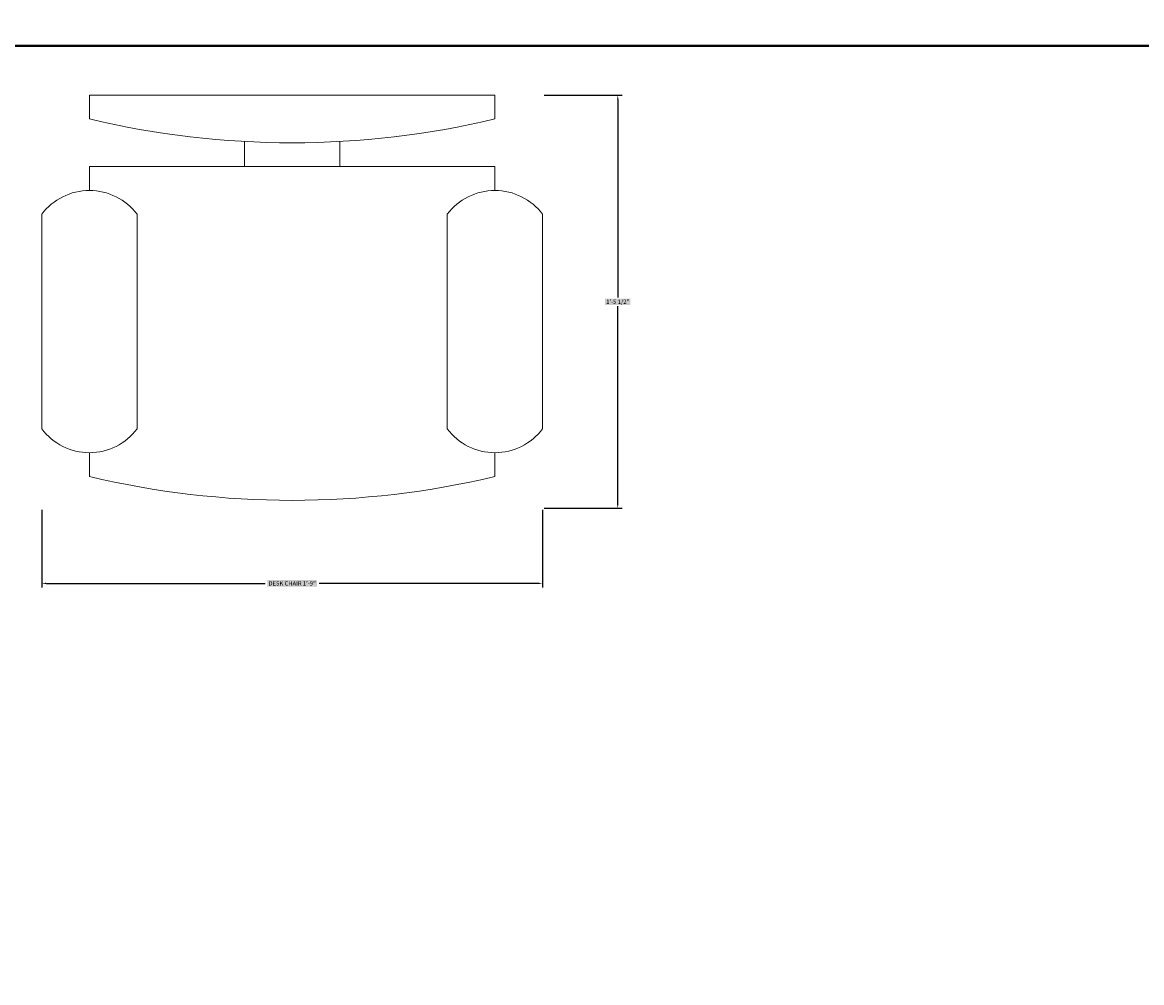
# Model space of a CAD drawing. Units: inches. Extents: x -301 to 715, y -607 to 364.
# Tile 76 of 141: x -170 to -123, y 26 to 67. Entities that reach past the tile are written whole.
import ezdxf

# ---------------------------------------------------------------- set-up
doc = ezdxf.new("R2010")
doc.units = ezdxf.units.IN
doc.header["$MEASUREMENT"] = 0
for name, color, linetype, lineweight in [('A-ANNO-DIMS', 2, 'Continuous', 18), ('A-FURN', 8, 'Continuous', 18), ('A-WALL', 3, 'Continuous', 40)]:
    doc.layers.add(name, color=color, linetype=linetype, lineweight=lineweight)
doc.styles.get("Standard").update_dxf_attribs({"font": 'arial.ttf'})
doc.dimstyles.get("Standard").update_dxf_attribs({"dimtxt": 0.18, "dimasz": 0.18, "dimexe": 0.18, "dimexo": 0.0625, "dimgap": 0.09, "dimtad": 0, "dimtih": 1, "dimtoh": 1, "dimdec": 1, "dimzin": 0, "dimdsep": 46, "dimlunit": 4, "dimtxsty": 'Standard', "dimcen": 0.09, "dimclrd": 3, "dimclre": 4, "dimclrt": 6, "dimadec": 0, "dimazin": 0, "dimtfac": 1, "dimtdec": 1, "dimtofl": 0, "dimtmove": 0, "dimatfit": 3, "dimfxl": 1, "dimtfill": 2, "dimtfillclr": 51, "dimtolj": 1, "dimtzin": 0, "dimarcsym": 0})

# ---------------------------------------------------------------- blocks, each defined once
blk = doc.blocks.new('Chair - Desk')
for p, q in [((-8.5, 0), (-8.5, -1)), ((-8.5, 0), (8.5, 0)), ((8.5, 0), (8.5, -1)), ((-2, -3), (-2, -1.9355)), ((2, -1.9576), (2, -3)), ((-8.5, -3), (-8.5, -4)), ((-8.5, -3), (8.5, -3)), ((8.5, -3), (8.5, -4)), ((-10.5, -5), (-10.5, -14)), ((-6.5, -14), (-6.5, -5)), ((6.5, -5), (6.5, -14)), ((10.5, -14), (10.5, -5)), ((-8.5, -15), (-8.5, -16)), ((8.5, -15), (8.5, -16))]:
    blk.add_line(p, q)
for centre, radius, start, end in [((0, 34.625), 36.625, 256.5803, 283.4197), ((-8.5, -6.5), 2.5, 36.8699, 143.1301), ((8.5, -6.5), 2.5, 36.8699, 143.1301), ((-8.5, -12.5), 2.5, 216.8699, 323.1301), ((8.5, -12.5), 2.5, 216.8699, 323.1301), ((0, 19.625), 36.625, 256.5803, 283.4197)]:
    blk.add_arc(centre, radius, start, end)
blk = doc.blocks.new('*D56')
at = {"layer": 'A-ANNO-DIMS', "color": 0, "lineweight": -2, "transparency": 16777216}
for p, q in [((-195.541, 65.682), (-172.295, 65.682)), ((-172.475, 60.682), (-172.475, 0.778)), ((-172.475, -62.318), (-172.475, -2.414)), ((-195.541, -67.318), (-172.295, -67.318))]:
    blk.add_line(p, q, dxfattribs=at)
at = {"layer": 'A-ANNO-DIMS', "color": 0, "transparency": 16777216}
for points in [[(-173.308, 60.682), (-171.641, 60.682), (-172.475, 65.682)], [(-173.308, -62.318), (-171.641, -62.318), (-172.475, -67.318)]]:
    blk.add_solid(points, dxfattribs=at)
at = {"layer": 'Defpoints', "color": 0, "transparency": 16777216}
for p in [(-195.603, 65.682), (-172.475, 65.682), (-195.603, -67.318)]:
    blk.add_point(p, dxfattribs=at)
at = {"layer": 'A-ANNO-DIMS', "color": 0, "transparency": 16777216, "insert": (-172.475, -0.818), "char_height": 3, "attachment_point": 5, "bg_fill": 1, "box_fill_scale": 1.25, "bg_fill_color": 51, "bg_fill_transparency": 0}
blk.add_mtext('\\A1;11\'-1"', dxfattribs=at)
blk = doc.blocks.new('*D136')
at = {"layer": 'A-ANNO-DIMS', "color": 4, "lineweight": -2, "transparency": 16777216}
for p, q in [((-169.593, 46.217), (-169.593, 42.95)), ((-148.593, 46.217), (-148.593, 42.95))]:
    blk.add_line(p, q, dxfattribs=at)
at = {"layer": 'A-ANNO-DIMS', "color": 3, "lineweight": -2, "transparency": 16777216}
for p, q in [((-169.413, 43.13), (-160.221, 43.13)), ((-148.773, 43.13), (-157.965, 43.13))]:
    blk.add_line(p, q, dxfattribs=at)
at = {"layer": 'A-ANNO-DIMS', "color": 3, "transparency": 16777216}
for points in [[(-169.413, 43.16), (-169.413, 43.1), (-169.593, 43.13)], [(-148.773, 43.16), (-148.773, 43.1), (-148.593, 43.13)]]:
    blk.add_solid(points, dxfattribs=at)
at = {"layer": 'Defpoints', "color": 0, "transparency": 16777216}
for p in [(-169.593, 46.28), (-148.593, 46.28), (-148.593, 43.13)]:
    blk.add_point(p, dxfattribs=at)
at = {"layer": 'A-ANNO-DIMS', "color": 6, "transparency": 16777216, "insert": (-159.093, 43.13), "char_height": 0.18, "attachment_point": 5, "bg_fill": 1, "box_fill_scale": 1.25, "bg_fill_color": 51, "bg_fill_transparency": 0}
blk.add_mtext('\\A1;DESK CHAIR 1\'-9"', dxfattribs=at)
blk = doc.blocks.new('*D137')
at = {"layer": 'A-ANNO-DIMS', "color": 4, "lineweight": -2, "transparency": 16777216}
for p, q in [((-148.53, 63.613), (-145.263, 63.613)), ((-148.53, 46.28), (-145.263, 46.28))]:
    blk.add_line(p, q, dxfattribs=at)
at = {"layer": 'A-ANNO-DIMS', "color": 3, "lineweight": -2, "transparency": 16777216}
for p, q in [((-145.443, 63.433), (-145.443, 55.129)), ((-145.443, 46.46), (-145.443, 54.763))]:
    blk.add_line(p, q, dxfattribs=at)
at = {"layer": 'A-ANNO-DIMS', "color": 3, "transparency": 16777216}
for points in [[(-145.473, 63.433), (-145.413, 63.433), (-145.443, 63.613)], [(-145.473, 46.46), (-145.413, 46.46), (-145.443, 46.28)]]:
    blk.add_solid(points, dxfattribs=at)
at = {"layer": 'Defpoints', "color": 0, "transparency": 16777216}
for p in [(-148.593, 63.613), (-145.443, 63.613), (-148.593, 46.28)]:
    blk.add_point(p, dxfattribs=at)
at = {"layer": 'A-ANNO-DIMS', "color": 6, "transparency": 16777216, "insert": (-145.443, 54.946), "char_height": 0.18, "attachment_point": 5, "bg_fill": 1, "box_fill_scale": 1.25, "bg_fill_color": 51, "bg_fill_transparency": 0}
blk.add_mtext('\\A1;1\'-5 1/2"', dxfattribs=at)
blk = doc.blocks.new('*D151')
at = {"layer": 'A-ANNO-DIMS', "color": 4, "lineweight": -2, "transparency": 16777216}
for p, q in [((-204.603, -223.755), (-204.603, 359.612)), ((-45.603, -214.755), (-45.603, 359.612))]:
    blk.add_line(p, q, dxfattribs=at)
at = {"layer": 'A-ANNO-DIMS', "color": 3, "lineweight": -2, "transparency": 16777216}
for p, q in [((-204.423, 359.432), (-125.494, 359.432)), ((-45.783, 359.432), (-124.713, 359.432))]:
    blk.add_line(p, q, dxfattribs=at)
at = {"layer": 'A-ANNO-DIMS', "color": 3, "transparency": 16777216}
for points in [[(-204.423, 359.462), (-204.423, 359.402), (-204.603, 359.432)], [(-45.783, 359.462), (-45.783, 359.402), (-45.603, 359.432)]]:
    blk.add_solid(points, dxfattribs=at)
at = {"layer": 'Defpoints', "color": 0, "transparency": 16777216}
for p in [(-45.603, 359.432), (-45.603, -214.818), (-204.603, -223.818)]:
    blk.add_point(p, dxfattribs=at)
at = {"layer": 'A-ANNO-DIMS', "color": 6, "transparency": 16777216, "insert": (-125.103, 359.432), "char_height": 0.18, "attachment_point": 5, "bg_fill": 1, "box_fill_scale": 1.25, "bg_fill_color": 51, "bg_fill_transparency": 0}
blk.add_mtext('\\A1;13\'-3"', dxfattribs=at)

msp = doc.modelspace()

# ---------------------------------------------------------------- linework, layer by layer
at = {"layer": 'A-WALL'}
msp.add_line((-45.603, 65.682), (-195.603, 65.682), dxfattribs=at)

# ---------------------------------------------------------------- block references
at = {"layer": 'A-FURN'}
msp.add_blockref('Chair - Desk', (-159.093, 63.613), dxfattribs=at)

# ---------------------------------------------------------------- dimensions: what is measured, and where the dimension line sits
at = {"layer": 'A-ANNO-DIMS'}
dim = msp.add_linear_dim(base=(-45.603, 359.432), p1=(-204.603, -223.818), p2=(-45.603, -214.818), dimstyle='Standard', override={"dimdec": 1, "dimlfac": 1, "dimrnd": 0, "dimzin": 1, "dimdsep": 46, "dimlunit": 4, "dimfrac": 2}, dxfattribs=at)
dim.commit()
dim.dimension.update_dxf_attribs({"geometry": '*D151', "text_midpoint": (-125.103, 359.432)})
for base, p1, p2, override, picture, middle in [((-172.475, 65.682), (-195.603, -67.318), (-195.603, 65.682), {"dimtxt": 3, "dimasz": 5, "dimclrd": 0, "dimclre": 0, "dimclrt": 0}, '*D56', (-172.475, -0.818)), ((-145.443, 63.613), (-148.593, 46.28), (-148.593, 63.613), {"dimdec": 1, "dimlfac": 1, "dimrnd": 0, "dimzin": 1, "dimdsep": 46, "dimlunit": 4, "dimfrac": 2}, '*D137', (-145.443, 54.946))]:
    dim = msp.add_linear_dim(base=base, p1=p1, p2=p2, angle=90, dimstyle='Standard', override=override, dxfattribs=at)
    dim.commit()
    dim.dimension.update_dxf_attribs({"geometry": picture, "text_midpoint": middle})
dim = msp.add_linear_dim(base=(-148.593, 43.13), p1=(-169.593, 46.28), p2=(-148.593, 46.28), text='DESK CHAIR <>', dimstyle='Standard', override={"dimdec": 1, "dimlfac": 1, "dimrnd": 0, "dimzin": 1, "dimdsep": 46, "dimlunit": 4, "dimfrac": 2}, dxfattribs=at)
dim.commit()
dim.dimension.update_dxf_attribs({"geometry": '*D136', "text_midpoint": (-159.093, 43.13)})

doc.saveas('drawing.dxf')
